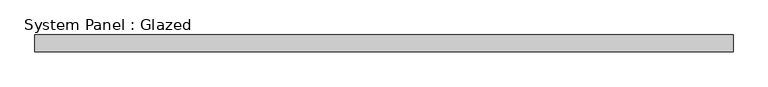
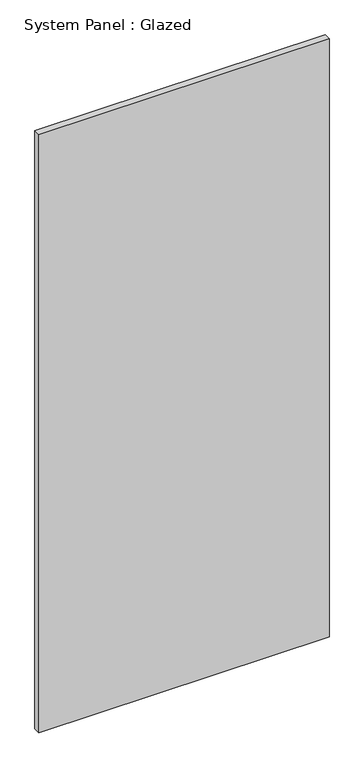
"""IFC4 building model written with IfcOpenShell, lengths in millimetres: plate geometry, System Panel : Glazed."""

from ifc_helpers import new_model, si_unit, origin, origin_with_axes, place, context, project, spatial, polyline, outline, extrude, source, transform, mapped, element, save


def system_panel_glazed_6ba90871(model_context):
    return source(origin(), model_context, "Body", "SweptSolid", [
        extrude(outline(polyline([(530.225, 19.05), (-530.225, 19.05), (-530.225, 44.45), (530.225, 44.45), (530.225, 19.05)])), origin_with_axes(), (0.0, 0.0, 1.0), 2311.4),
    ])


if __name__ == "__main__":
    model = new_model("IFC4")
    model_context = context("Model", 3, world=origin())
    ifc_project = project(units=[si_unit("LENGTHUNIT", "METRE", prefix="MILLI")], contexts=[model_context])
    site = spatial("IfcSite", under=ifc_project)
    building = spatial("IfcBuilding", under=site)
    placement = place(None, origin())
    system_panel_glazed_shape = system_panel_glazed_6ba90871(model_context)
    element("IfcPlate", 1, ObjectType="System Panel : Glazed", at=placement, inside=building, context=model_context, shape_type="MappedRepresentation", body=[
        mapped(system_panel_glazed_shape, transform((0.0, 0.0, 0.0), x_axis=(1.0, 0.0, 0.0), y_axis=(0.0, 1.0, 0.0), z_axis=(0.0, 0.0, 1.0))),
    ])
    save(model, "model.ifc")

# Revit data of these elements
# Type "System Panel : Glazed"
#   Construction Type Id = "GSP4R"
#   Analytic Construction = "1/8 in Pilkington single glazing"
#   Visual Light Transmittance = 0.9
#   Solar Heat Gain Coefficient = 0.86
#   Heat Transfer Coefficient (U) = 1.18115 BTU/(h·ft²·°F)
#   Define Thermal Properties by = 1
# Element 1 (IfcPlate, "System Panel : Glazed")
#   Materials on its faces: "Glass"
# Materials
#   "Glass": class "Glass", colour RGB 0 128 192, transparency 0.75, Description = "Soda Lime Glass", Cost = 0
